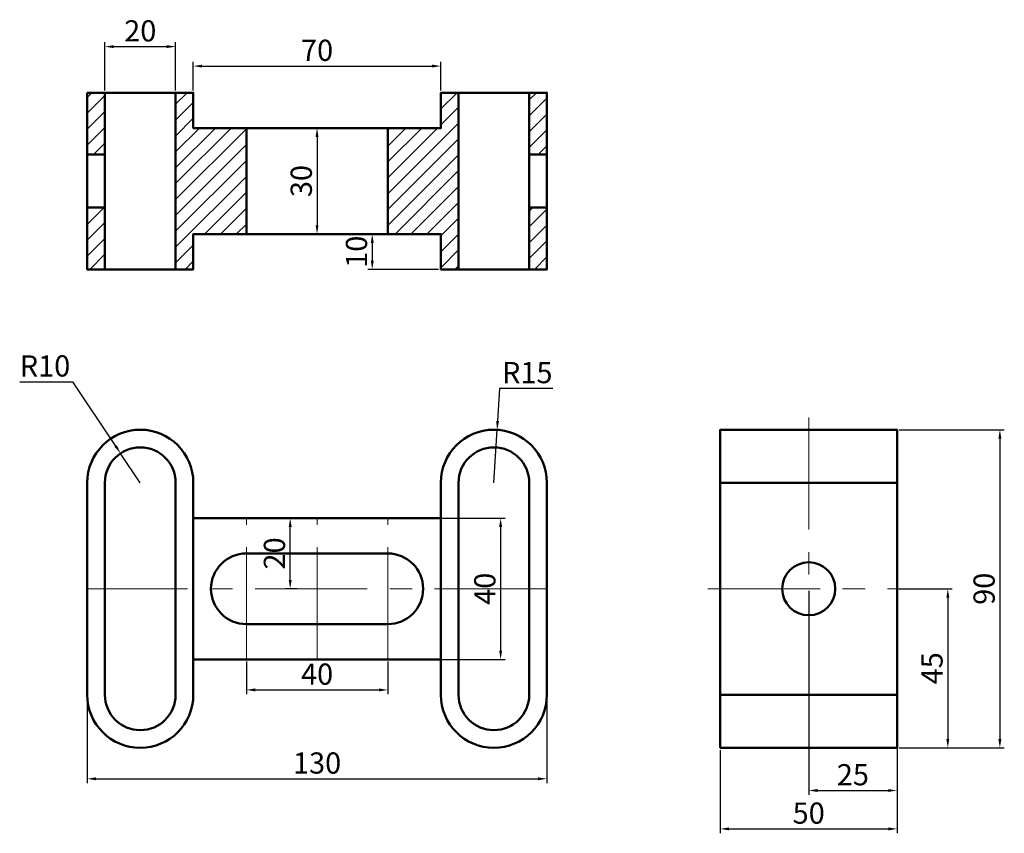
# Model space of a CAD drawing. Units: millimetres. Extents: x 12 to 290, y 11 to 241.
import ezdxf

# ---------------------------------------------------------------- set-up
doc = ezdxf.new("R2010")
doc.units = ezdxf.units.MM
doc.linetypes.add('CENTER', pattern=[50.8, 31.75, -6.35, 6.35, -6.35])
for name, color, linetype, lineweight in [('M-CNTR', 1, 'CENTER', 18), ('M-DIMS', 2, 'Continuous', 25), ('M-HATC', 8, 'Continuous', 18), ('M-OUTL', 7, 'Continuous', 50)]:
    doc.layers.add(name, color=color, linetype=linetype, lineweight=lineweight)
doc.styles.get("Standard").update_dxf_attribs({"font": 'arial.ttf'})
doc.dimstyles.new('ISO-25', dxfattribs={"dimtxt": 6, "dimasz": 2.5, "dimexe": 1.25, "dimexo": 0.625, "dimtad": 1, "dimtoh": 1, "dimdec": 0, "dimtxsty": 'Standard', "dimcen": 2.5, "dimadec": 0, "dimazin": 0, "dimtfac": 1, "dimtdec": 0, "dimtmove": 0, "dimatfit": 3, "dimfxl": 1, "dimarcsym": 0})

# ---------------------------------------------------------------- blocks, each defined once
blk = doc.blocks.new('*D1')
at = {"layer": 'Defpoints', "color": 0, "transparency": 16777216}
for p in [(130.72, 180.64), (111.32, 170.64), (130.72, 170.64)]:
    blk.add_point(p, dxfattribs=at)
at = {"layer": 'M-DIMS', "color": 0, "lineweight": -2, "transparency": 16777216}
for p, q in [((130.09, 180.64), (110.07, 180.64)), ((111.32, 178.14), (111.32, 173.14)), ((130.09, 170.64), (110.07, 170.64))]:
    blk.add_line(p, q, dxfattribs=at)
at = {"layer": 'M-DIMS', "color": 0, "transparency": 16777216}
for points in [[(110.91, 178.14), (111.74, 178.14), (111.32, 180.64)], [(110.91, 173.14), (111.74, 173.14), (111.32, 170.64)]]:
    blk.add_solid(points, dxfattribs=at)
at = {"layer": 'M-DIMS', "color": 0, "transparency": 16777216, "insert": (107.64, 175.64), "char_height": 6, "attachment_point": 5, "rotation": 90}
blk.add_mtext('10', dxfattribs=at)
blk = doc.blocks.new('*D2')
at = {"layer": 'Defpoints', "color": 0, "transparency": 16777216}
for p in [(55.72, 233.67), (35.72, 220.64), (55.72, 220.64)]:
    blk.add_point(p, dxfattribs=at)
at = {"layer": 'M-DIMS', "color": 0, "lineweight": -2, "transparency": 16777216}
for p, q in [((35.72, 221.26), (35.72, 234.92)), ((55.72, 221.26), (55.72, 234.92)), ((38.22, 233.67), (53.22, 233.67))]:
    blk.add_line(p, q, dxfattribs=at)
at = {"layer": 'M-DIMS', "color": 0, "transparency": 16777216}
for points in [[(38.22, 234.09), (38.22, 233.25), (35.72, 233.67)], [(53.22, 234.09), (53.22, 233.25), (55.72, 233.67)]]:
    blk.add_solid(points, dxfattribs=at)
at = {"layer": 'M-DIMS', "color": 0, "transparency": 16777216, "insert": (45.72, 237.36), "char_height": 6, "attachment_point": 5}
blk.add_mtext('20', dxfattribs=at)
blk = doc.blocks.new('*D3')
at = {"layer": 'Defpoints', "color": 0, "transparency": 16777216}
for p in [(130.72, 228.16), (60.72, 220.64), (130.72, 220.64)]:
    blk.add_point(p, dxfattribs=at)
at = {"layer": 'M-DIMS', "color": 0, "lineweight": -2, "transparency": 16777216}
for p, q in [((60.72, 221.26), (60.72, 229.41)), ((130.72, 221.26), (130.72, 229.41)), ((63.22, 228.16), (128.22, 228.16))]:
    blk.add_line(p, q, dxfattribs=at)
at = {"layer": 'M-DIMS', "color": 0, "transparency": 16777216}
for points in [[(63.22, 228.58), (63.22, 227.75), (60.72, 228.16)], [(128.22, 228.58), (128.22, 227.75), (130.72, 228.16)]]:
    blk.add_solid(points, dxfattribs=at)
at = {"layer": 'M-DIMS', "color": 0, "transparency": 16777216, "insert": (95.72, 231.85), "char_height": 6, "attachment_point": 5}
blk.add_mtext('70', dxfattribs=at)
blk = doc.blocks.new('*D4')
at = {"layer": 'Defpoints', "color": 0, "transparency": 16777216}
for p in [(95.72, 210.64), (95.72, 180.64), (95.72, 180.64)]:
    blk.add_point(p, dxfattribs=at)
at = {"layer": 'M-DIMS', "color": 0, "lineweight": -2, "transparency": 16777216}
for p, q in [((96.34, 210.64), (96.97, 210.64)), ((95.72, 208.14), (95.72, 183.14)), ((96.34, 180.64), (96.97, 180.64))]:
    blk.add_line(p, q, dxfattribs=at)
at = {"layer": 'M-DIMS', "color": 0, "transparency": 16777216}
for points in [[(95.3, 208.14), (96.13, 208.14), (95.72, 210.64)], [(95.3, 183.14), (96.13, 183.14), (95.72, 180.64)]]:
    blk.add_solid(points, dxfattribs=at)
at = {"layer": 'M-DIMS', "color": 0, "transparency": 16777216, "insert": (92.03, 195.64), "char_height": 6, "attachment_point": 5, "rotation": 90}
blk.add_mtext('30', dxfattribs=at)
blk = doc.blocks.new('*D5')
at = {"layer": 'Defpoints', "color": 0, "transparency": 16777216}
for p in [(146.63, 125.25), (145.72, 110.28)]:
    blk.add_point(p, dxfattribs=at)
at = {"layer": 'M-DIMS', "color": 0, "lineweight": -2, "transparency": 16777216}
for p, q in [((147.34, 136.98), (146.78, 127.75)), ((162.35, 136.98), (147.34, 136.98)), ((145.72, 110.28), (146.63, 125.25))]:
    blk.add_line(p, q, dxfattribs=at)
at = {"layer": 'M-DIMS', "color": 0, "transparency": 16777216}
blk.add_solid([(146.36, 127.77), (147.2, 127.72), (146.63, 125.25)], dxfattribs=at)
at = {"layer": 'M-DIMS', "color": 0, "transparency": 16777216, "insert": (155.16, 140.67), "char_height": 6, "attachment_point": 5}
blk.add_mtext('R15', dxfattribs=at)
blk = doc.blocks.new('*D6')
at = {"layer": 'Defpoints', "color": 0, "transparency": 16777216}
for p in [(40.15, 118.59), (45.72, 110.28)]:
    blk.add_point(p, dxfattribs=at)
at = {"layer": 'M-DIMS', "color": 0, "lineweight": -2, "transparency": 16777216}
for p, q in [((11.62, 138.86), (26.56, 138.86)), ((26.56, 138.86), (38.76, 120.67)), ((45.72, 110.28), (40.15, 118.59))]:
    blk.add_line(p, q, dxfattribs=at)
at = {"layer": 'M-DIMS', "color": 0, "transparency": 16777216}
blk.add_solid([(39.1, 120.9), (38.41, 120.43), (40.15, 118.59)], dxfattribs=at)
at = {"layer": 'M-DIMS', "color": 0, "transparency": 16777216, "insert": (18.78, 142.55), "char_height": 6, "attachment_point": 5}
blk.add_mtext('R10', dxfattribs=at)
blk = doc.blocks.new('*D7')
at = {"layer": 'Defpoints', "color": 0, "transparency": 16777216}
for p in [(88.12, 100.28), (90.72, 100.28), (90.72, 80.28)]:
    blk.add_point(p, dxfattribs=at)
at = {"layer": 'M-DIMS', "color": 0, "lineweight": -2, "transparency": 16777216}
for p, q in [((90.09, 100.28), (86.87, 100.28)), ((88.12, 82.78), (88.12, 97.78)), ((90.09, 80.28), (86.87, 80.28))]:
    blk.add_line(p, q, dxfattribs=at)
at = {"layer": 'M-DIMS', "color": 0, "transparency": 16777216}
for points in [[(87.7, 97.78), (88.54, 97.78), (88.12, 100.28)], [(87.7, 82.78), (88.54, 82.78), (88.12, 80.28)]]:
    blk.add_solid(points, dxfattribs=at)
at = {"layer": 'M-DIMS', "color": 0, "transparency": 16777216, "insert": (84.43, 90.28), "char_height": 6, "attachment_point": 5, "rotation": 90}
blk.add_mtext('20', dxfattribs=at)
blk = doc.blocks.new('*D8')
at = {"layer": 'Defpoints', "color": 0, "transparency": 16777216}
for p in [(75.72, 60.28), (115.72, 60.28), (115.72, 51.67)]:
    blk.add_point(p, dxfattribs=at)
at = {"layer": 'M-DIMS', "color": 0, "lineweight": -2, "transparency": 16777216}
for p, q in [((75.72, 59.66), (75.72, 50.42)), ((115.72, 59.66), (115.72, 50.42)), ((78.22, 51.67), (113.22, 51.67))]:
    blk.add_line(p, q, dxfattribs=at)
at = {"layer": 'M-DIMS', "color": 0, "transparency": 16777216}
for points in [[(78.22, 52.09), (78.22, 51.25), (75.72, 51.67)], [(113.22, 52.09), (113.22, 51.25), (115.72, 51.67)]]:
    blk.add_solid(points, dxfattribs=at)
at = {"layer": 'M-DIMS', "color": 0, "transparency": 16777216, "insert": (95.72, 55.36), "char_height": 6, "attachment_point": 5}
blk.add_mtext('40', dxfattribs=at)
blk = doc.blocks.new('*D9')
at = {"layer": 'Defpoints', "color": 0, "transparency": 16777216}
for p in [(115.72, 100.28), (115.72, 60.28), (147.63, 60.28)]:
    blk.add_point(p, dxfattribs=at)
at = {"layer": 'M-DIMS', "color": 0, "lineweight": -2, "transparency": 16777216}
for p, q in [((116.34, 100.28), (148.88, 100.28)), ((147.63, 97.78), (147.63, 62.78)), ((116.34, 60.28), (148.88, 60.28))]:
    blk.add_line(p, q, dxfattribs=at)
at = {"layer": 'M-DIMS', "color": 0, "transparency": 16777216}
for points in [[(147.21, 97.78), (148.05, 97.78), (147.63, 100.28)], [(147.21, 62.78), (148.05, 62.78), (147.63, 60.28)]]:
    blk.add_solid(points, dxfattribs=at)
at = {"layer": 'M-DIMS', "color": 0, "transparency": 16777216, "insert": (143.94, 80.28), "char_height": 6, "attachment_point": 5, "rotation": 90}
blk.add_mtext('40', dxfattribs=at)
blk = doc.blocks.new('*D10')
at = {"layer": 'Defpoints', "color": 0, "transparency": 16777216}
for p in [(259.75, 125.28), (259.75, 35.28), (288.82, 35.28)]:
    blk.add_point(p, dxfattribs=at)
at = {"layer": 'M-DIMS', "color": 0, "lineweight": -2, "transparency": 16777216}
for p, q in [((260.38, 125.28), (290.07, 125.28)), ((288.82, 122.78), (288.82, 37.78)), ((260.38, 35.28), (290.07, 35.28))]:
    blk.add_line(p, q, dxfattribs=at)
at = {"layer": 'M-DIMS', "color": 0, "transparency": 16777216}
for points in [[(288.4, 122.78), (289.24, 122.78), (288.82, 125.28)], [(288.4, 37.78), (289.24, 37.78), (288.82, 35.28)]]:
    blk.add_solid(points, dxfattribs=at)
at = {"layer": 'M-DIMS', "color": 0, "transparency": 16777216, "insert": (285.13, 80.28), "char_height": 6, "attachment_point": 5, "rotation": 90}
blk.add_mtext('90', dxfattribs=at)
blk = doc.blocks.new('*D11')
at = {"layer": 'Defpoints', "color": 0, "transparency": 16777216}
for p in [(259.75, 80.28), (259.75, 35.28), (274.09, 35.28)]:
    blk.add_point(p, dxfattribs=at)
at = {"layer": 'M-DIMS', "color": 0, "lineweight": -2, "transparency": 16777216}
for p, q in [((260.38, 80.28), (275.34, 80.28)), ((274.09, 77.78), (274.09, 37.78)), ((260.38, 35.28), (275.34, 35.28))]:
    blk.add_line(p, q, dxfattribs=at)
at = {"layer": 'M-DIMS', "color": 0, "transparency": 16777216}
for points in [[(273.67, 77.78), (274.5, 77.78), (274.09, 80.28)], [(273.67, 37.78), (274.5, 37.78), (274.09, 35.28)]]:
    blk.add_solid(points, dxfattribs=at)
at = {"layer": 'M-DIMS', "color": 0, "transparency": 16777216, "insert": (270.41, 57.78), "char_height": 6, "attachment_point": 5, "rotation": 90}
blk.add_mtext('45', dxfattribs=at)
blk = doc.blocks.new('*D12')
at = {"layer": 'Defpoints', "color": 0, "transparency": 16777216}
for p in [(30.72, 50.28), (160.72, 50.28), (160.72, 26.51)]:
    blk.add_point(p, dxfattribs=at)
at = {"layer": 'M-DIMS', "color": 0, "lineweight": -2, "transparency": 16777216}
for p, q in [((30.72, 49.66), (30.72, 25.26)), ((160.72, 49.66), (160.72, 25.26)), ((33.22, 26.51), (158.22, 26.51))]:
    blk.add_line(p, q, dxfattribs=at)
at = {"layer": 'M-DIMS', "color": 0, "transparency": 16777216}
for points in [[(33.22, 26.93), (33.22, 26.1), (30.72, 26.51)], [(158.22, 26.93), (158.22, 26.1), (160.72, 26.51)]]:
    blk.add_solid(points, dxfattribs=at)
at = {"layer": 'M-DIMS', "color": 0, "transparency": 16777216, "insert": (95.72, 30.2), "char_height": 6, "attachment_point": 5}
blk.add_mtext('130', dxfattribs=at)
blk = doc.blocks.new('*D13')
at = {"layer": 'Defpoints', "color": 0, "transparency": 16777216}
for p in [(209.75, 35.28), (259.75, 35.28), (259.75, 12.34)]:
    blk.add_point(p, dxfattribs=at)
at = {"layer": 'M-DIMS', "color": 0, "lineweight": -2, "transparency": 16777216}
for p, q in [((209.75, 34.66), (209.75, 11.09)), ((259.75, 34.66), (259.75, 11.09)), ((212.25, 12.34), (257.25, 12.34))]:
    blk.add_line(p, q, dxfattribs=at)
at = {"layer": 'M-DIMS', "color": 0, "transparency": 16777216}
for points in [[(212.25, 12.76), (212.25, 11.92), (209.75, 12.34)], [(257.25, 12.76), (257.25, 11.92), (259.75, 12.34)]]:
    blk.add_solid(points, dxfattribs=at)
at = {"layer": 'M-DIMS', "color": 0, "transparency": 16777216, "insert": (234.75, 16.03), "char_height": 6, "attachment_point": 5}
blk.add_mtext('50', dxfattribs=at)
blk = doc.blocks.new('*D14')
at = {"layer": 'Defpoints', "color": 0, "transparency": 16777216}
for p in [(234.75, 80.28), (259.75, 80.28), (259.75, 23.21)]:
    blk.add_point(p, dxfattribs=at)
at = {"layer": 'M-DIMS', "color": 0, "lineweight": -2, "transparency": 16777216}
for p, q in [((234.75, 79.66), (234.75, 21.96)), ((259.75, 79.66), (259.75, 21.96)), ((237.25, 23.21), (257.25, 23.21))]:
    blk.add_line(p, q, dxfattribs=at)
at = {"layer": 'M-DIMS', "color": 0, "transparency": 16777216}
for points in [[(237.25, 23.62), (237.25, 22.79), (234.75, 23.21)], [(257.25, 23.62), (257.25, 22.79), (259.75, 23.21)]]:
    blk.add_solid(points, dxfattribs=at)
at = {"layer": 'M-DIMS', "color": 0, "transparency": 16777216, "insert": (247.25, 26.89), "char_height": 6, "attachment_point": 5}
blk.add_mtext('25', dxfattribs=at)

msp = doc.modelspace()

# ---------------------------------------------------------------- hatches: boundary and pattern name
at = {"layer": 'M-HATC'}
h = msp.add_hatch(dxfattribs=at)
h.set_pattern_fill('ANSI31', color=256)
h.paths.add_polyline_path([(35.72, 220.64), (30.72, 220.64), (30.72, 203.14), (35.72, 203.14)])
h.paths.add_polyline_path([(35.72, 188.14), (30.72, 188.14), (30.72, 170.64), (35.72, 170.64)])
h.paths.add_polyline_path([(75.72, 210.64), (60.72, 210.64), (60.72, 220.64), (55.72, 220.64), (55.72, 170.64), (60.72, 170.64), (60.72, 180.64), (75.72, 180.64)])
h.paths.add_polyline_path([(135.72, 220.64), (130.72, 220.64), (130.72, 210.64), (115.72, 210.64), (115.72, 180.64), (130.72, 180.64), (130.72, 170.64), (135.72, 170.64)])
h.paths.add_polyline_path([(160.72, 220.64), (155.72, 220.64), (155.72, 203.14), (160.72, 203.14)])
h.paths.add_polyline_path([(160.72, 188.14), (155.72, 188.14), (155.72, 170.64), (160.72, 170.64)])

# ---------------------------------------------------------------- linework, layer by layer
at = {"layer": 'M-CNTR'}
for p, q in [((234.75, 128.78), (234.75, 31.78)), ((75.72, 60.28), (75.72, 100.28)), ((95.72, 60.28), (95.72, 100.28)), ((115.72, 60.28), (115.72, 100.28)), ((160.72, 80.28), (30.72, 80.28)), ((206.25, 80.28), (263.25, 80.28))]:
    msp.add_line(p, q, dxfattribs=at)
at = {"layer": 'M-OUTL'}
for p, q in [((35.72, 170.64), (35.72, 220.64)), ((55.72, 170.64), (55.72, 220.64)), ((135.72, 220.64), (135.72, 170.64)), ((155.72, 220.64), (155.72, 170.64)), ((75.72, 180.64), (75.72, 210.64)), ((115.72, 180.64), (115.72, 210.64)), ((30.72, 203.14), (35.72, 203.14)), ((160.72, 203.14), (155.72, 203.14)), ((30.72, 188.14), (35.72, 188.14)), ((160.72, 188.14), (155.72, 188.14)), ((209.75, 110.28), (259.75, 110.28)), ((130.72, 100.28), (60.72, 100.28)), ((130.72, 60.28), (60.72, 60.28)), ((209.75, 50.28), (259.75, 50.28))]:
    msp.add_line(p, q, dxfattribs=at)
for points in [[(30.72, 220.64), (60.72, 220.64), (60.72, 210.64), (130.72, 210.64), (130.72, 220.64), (160.72, 220.64), (160.72, 170.64), (130.72, 170.64), (130.72, 180.64), (60.72, 180.64), (60.72, 170.64), (30.72, 170.64)], [(259.75, 35.28), (259.75, 125.28), (209.75, 125.28), (209.75, 35.28)]]:
    msp.add_lwpolyline(points, close=True, dxfattribs=at)
for points in [[(60.72, 110.28), (60.72, 50.28, -1), (30.72, 50.28), (30.72, 110.28, -1)], [(160.72, 110.28), (160.72, 50.28, -1), (130.72, 50.28), (130.72, 110.28, -1)], [(55.72, 110.28), (55.72, 50.28, -1), (35.72, 50.28), (35.72, 110.28, -1)], [(155.72, 110.28), (155.72, 50.28, -1), (135.72, 50.28), (135.72, 110.28, -1)], [(75.72, 70.28), (115.72, 70.28, 1), (115.72, 90.28), (75.72, 90.28, 1)]]:
    msp.add_lwpolyline(points, format="xyb", close=True, dxfattribs=at)
msp.add_circle((234.75, 80.28), 7.5, dxfattribs=at)

# ---------------------------------------------------------------- dimensions: what is measured, and where the dimension line sits
at = {"layer": 'M-DIMS'}
for base, p1, p2, picture, middle in [((55.72, 233.67), (35.72, 220.64), (55.72, 220.64), '*D2', (45.72, 237.36)), ((130.72, 228.16), (60.72, 220.64), (130.72, 220.64), '*D3', (95.72, 231.85)), ((259.75, 23.21), (234.75, 80.28), (259.75, 80.28), '*D14', (247.25, 26.89)), ((115.72, 51.67), (75.72, 60.28), (115.72, 60.28), '*D8', (95.72, 55.36)), ((160.72, 26.51), (30.72, 50.28), (160.72, 50.28), '*D12', (95.72, 30.2)), ((259.75, 12.34), (209.75, 35.28), (259.75, 35.28), '*D13', (234.75, 16.03))]:
    dim = msp.add_linear_dim(base=base, p1=p1, p2=p2, dimstyle='ISO-25', override={"dimclrd": 0, "dimclre": 0, "dimclrt": 0}, dxfattribs=at)
    dim.commit()
    dim.dimension.update_dxf_attribs({"geometry": picture, "text_midpoint": middle})
for base, p1, p2, picture, middle in [((95.72, 180.64), (95.72, 210.64), (95.72, 180.64), '*D4', (92.03, 195.64)), ((111.32, 170.64), (130.72, 180.64), (130.72, 170.64), '*D1', (107.64, 175.64)), ((288.82, 35.28), (259.75, 125.28), (259.75, 35.28), '*D10', (285.13, 80.28)), ((88.12, 100.28), (90.72, 80.28), (90.72, 100.28), '*D7', (84.43, 90.28)), ((147.63, 60.28), (115.72, 100.28), (115.72, 60.28), '*D9', (143.94, 80.28)), ((274.09, 35.28), (259.75, 80.28), (259.75, 35.28), '*D11', (270.41, 57.78))]:
    dim = msp.add_linear_dim(base=base, p1=p1, p2=p2, angle=90, dimstyle='ISO-25', override={"dimclrd": 0, "dimclre": 0, "dimclrt": 0}, dxfattribs=at)
    dim.commit()
    dim.dimension.update_dxf_attribs({"geometry": picture, "text_midpoint": middle})
for center, mpoint, picture, middle in [((45.72, 110.28), (40.15, 118.59), '*D6', (18.78, 138.86)), ((145.72, 110.28), (146.63, 125.25), '*D5', (155.16, 136.98))]:
    dim = msp.add_radius_dim(center=center, mpoint=mpoint, dimstyle='ISO-25', override={"dimclrd": 0, "dimclre": 0, "dimclrt": 0}, dxfattribs=at)
    dim.commit()
    dim.dimension.update_dxf_attribs({"geometry": picture, "text_midpoint": middle, "dimtype": 164})

doc.saveas('drawing.dxf')
